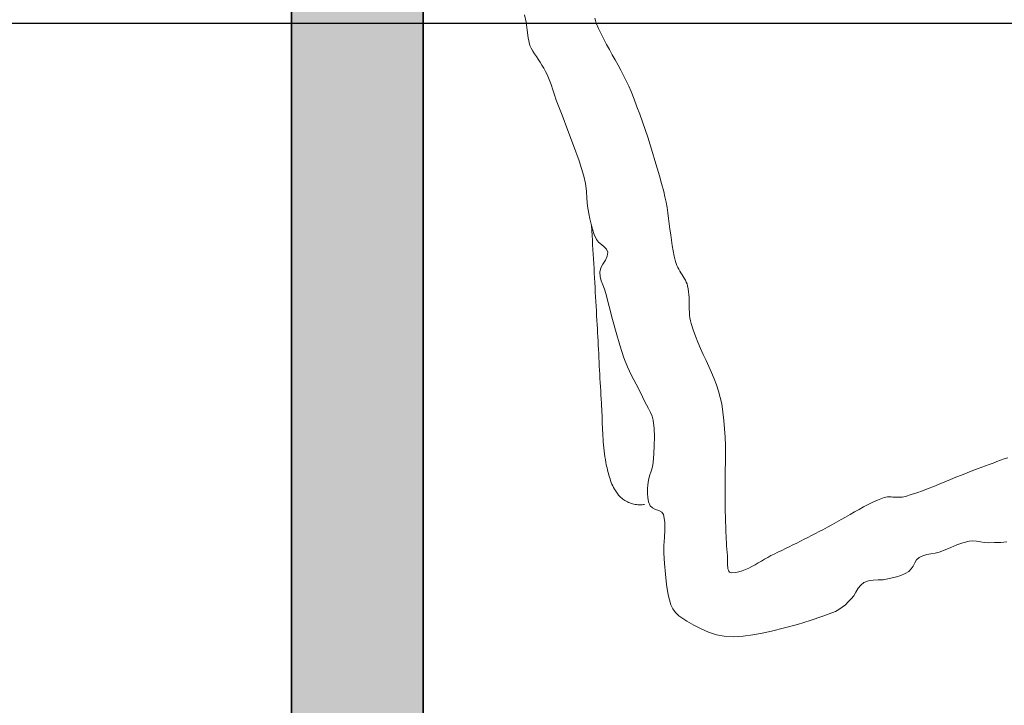
# Model space of a CAD drawing. Units: inches. Extents: x 2656 to 9931, y 1941 to 3068.
# Tile 15 of 46: x 2863 to 2896, y 2466 to 2490. Entities that reach past the tile are written whole.
import ezdxf

# ---------------------------------------------------------------- set-up
doc = ezdxf.new("R2010")
doc.units = ezdxf.units.IN
for name, color, linetype, lineweight in [('A-ANNO-DIMS', 2, 'Continuous', 18), ('A-FURN', 8, 'Continuous', 13), ('A-WALL', 7, 'Continuous', 35), ('A-WALL-PATT', 251, 'Continuous', 13)]:
    doc.layers.add(name, color=color, linetype=linetype, lineweight=lineweight)
doc.styles.get("Standard").update_dxf_attribs({"font": 'arial.ttf'})
doc.dimstyles.new('ISO-25', dxfattribs={"dimtxt": 6, "dimasz": 2.5, "dimexe": 1.25, "dimexo": 0.625, "dimtad": 1, "dimdec": 0, "dimlunit": 3, "dimtxsty": 'Standard', "dimcen": 2.5, "dimadec": 0, "dimazin": 0, "dimtfac": 1, "dimtdec": 0, "dimtmove": 0, "dimatfit": 3, "dimfxl": 1, "dimarcsym": 0})

# ---------------------------------------------------------------- blocks, each defined once
blk = doc.blocks.new('BED-DOUBLE')
for p, q in [((2.814, 22.253), (2.758, 22.509)), ((2.848, 21.988), (2.814, 22.253)), ((5.181, 22.309), (5.16, 22.395)), ((5.21, 22.225), (5.181, 22.309)), ((5.29, 22.04), (5.21, 22.225)), ((2.883, 21.722), (2.848, 21.988)), ((5.376, 21.857), (5.29, 22.04)), ((5.467, 21.676), (5.376, 21.857)), ((2.944, 21.465), (2.883, 21.722)), ((5.562, 21.498), (5.467, 21.676)), ((2.987, 21.364), (2.944, 21.465)), ((3.042, 21.269), (2.987, 21.364)), ((3.105, 21.176), (3.042, 21.269)), ((5.659, 21.32), (5.562, 21.498)), ((5.758, 21.144), (5.659, 21.32)), ((3.17, 21.085), (3.105, 21.176)), ((3.23, 20.991), (3.17, 21.085)), ((3.294, 20.888), (3.23, 20.991)), ((3.358, 20.785), (3.294, 20.888)), ((5.858, 20.967), (5.758, 21.144)), ((5.956, 20.79), (5.858, 20.967)), ((3.422, 20.681), (3.358, 20.785)), ((3.482, 20.575), (3.422, 20.681)), ((3.535, 20.466), (3.482, 20.575)), ((6.053, 20.612), (5.956, 20.79)), ((6.147, 20.433), (6.053, 20.612)), ((3.605, 20.296), (3.535, 20.466)), ((3.669, 20.123), (3.605, 20.296)), ((6.237, 20.253), (6.147, 20.433)), ((6.322, 20.069), (6.237, 20.253)), ((3.729, 19.948), (3.669, 20.123)), ((3.787, 19.772), (3.729, 19.948)), ((6.401, 19.883), (6.322, 20.069)), ((6.502, 19.627), (6.401, 19.883)), ((3.848, 19.598), (3.787, 19.772)), ((4.042, 19.079), (3.848, 19.598)), ((6.6, 19.369), (6.502, 19.627)), ((6.696, 19.11), (6.6, 19.369)), ((4.241, 18.561), (4.042, 19.079)), ((6.789, 18.85), (6.696, 19.11)), ((6.88, 18.59), (6.789, 18.85)), ((4.437, 18.043), (4.241, 18.561)), ((6.968, 18.328), (6.88, 18.59)), ((7.053, 18.065), (6.968, 18.328)), ((4.623, 17.521), (4.437, 18.043)), ((7.136, 17.802), (7.053, 18.065)), ((4.788, 16.993), (4.623, 17.521)), ((7.217, 17.538), (7.136, 17.802)), ((7.295, 17.273), (7.217, 17.538)), ((7.37, 17.008), (7.295, 17.273)), ((4.842, 16.744), (4.788, 16.993)), ((7.443, 16.742), (7.37, 17.008)), ((4.873, 16.49), (4.842, 16.744)), ((4.894, 16.234), (4.873, 16.49)), ((7.514, 16.475), (7.443, 16.742)), ((7.558, 16.293), (7.514, 16.475)), ((4.918, 15.978), (4.894, 16.234)), ((7.596, 16.111), (7.558, 16.293)), ((4.956, 15.726), (4.918, 15.978)), ((7.628, 15.927), (7.596, 16.111)), ((7.656, 15.742), (7.628, 15.927)), ((4.993, 15.544), (4.956, 15.726)), ((5.035, 15.362), (4.993, 15.544)), ((7.682, 15.557), (7.656, 15.742)), ((7.706, 15.371), (7.682, 15.557)), ((5.084, 15.183), (5.035, 15.362)), ((5.061, 15.137), (5.052, 15.298)), ((5.071, 14.976), (5.061, 15.137)), ((5.144, 15.008), (5.084, 15.183)), ((7.729, 15.185), (7.706, 15.371)), ((7.753, 14.999), (7.729, 15.185)), ((5.08, 14.815), (5.071, 14.976)), ((5.089, 14.653), (5.08, 14.815)), ((5.218, 14.839), (5.144, 15.008)), ((5.29, 14.745), (5.218, 14.839)), ((7.778, 14.814), (7.753, 14.999)), ((7.806, 14.629), (7.778, 14.814)), ((5.098, 14.492), (5.089, 14.653)), ((5.107, 14.331), (5.098, 14.492)), ((5.386, 14.665), (5.29, 14.745)), ((5.486, 14.589), (5.386, 14.665)), ((5.567, 14.505), (5.486, 14.589)), ((5.607, 14.402), (5.567, 14.505)), ((7.837, 14.445), (7.806, 14.629)), ((5.116, 14.17), (5.107, 14.331)), ((5.125, 14.008), (5.116, 14.17)), ((5.44, 13.998), (5.524, 14.129)), ((5.524, 14.129), (5.588, 14.261)), ((5.588, 14.261), (5.607, 14.402)), ((7.874, 14.262), (7.837, 14.445)), ((7.916, 14.08), (7.874, 14.262)), ((5.135, 13.847), (5.125, 14.008)), ((5.144, 13.686), (5.135, 13.847)), ((5.331, 13.725), (5.367, 13.865)), ((5.367, 13.865), (5.44, 13.998)), ((7.937, 14.012), (7.916, 14.08)), ((7.963, 13.946), (7.937, 14.012)), ((7.994, 13.881), (7.963, 13.946)), ((8.029, 13.818), (7.994, 13.881)), ((8.066, 13.756), (8.029, 13.818)), ((5.153, 13.525), (5.144, 13.686)), ((5.162, 13.363), (5.153, 13.525)), ((5.341, 13.575), (5.331, 13.725)), ((5.379, 13.427), (5.341, 13.575)), ((8.105, 13.695), (8.066, 13.756)), ((8.144, 13.633), (8.105, 13.695)), ((8.182, 13.572), (8.144, 13.633)), ((8.219, 13.51), (8.182, 13.572)), ((8.254, 13.447), (8.219, 13.51)), ((5.171, 13.202), (5.162, 13.363)), ((5.18, 13.041), (5.171, 13.202)), ((5.432, 13.282), (5.379, 13.427)), ((5.489, 13.137), (5.432, 13.282)), ((5.538, 12.991), (5.489, 13.137)), ((8.285, 13.382), (8.254, 13.447)), ((8.311, 13.316), (8.285, 13.382)), ((8.332, 13.248), (8.311, 13.316)), ((8.352, 13.151), (8.332, 13.248)), ((8.367, 13.053), (8.352, 13.151)), ((5.189, 12.88), (5.18, 13.041)), ((5.198, 12.718), (5.189, 12.88)), ((5.657, 12.549), (5.538, 12.991)), ((8.376, 12.954), (8.367, 13.053)), ((8.381, 12.855), (8.376, 12.954)), ((8.383, 12.755), (8.381, 12.855)), ((5.207, 12.557), (5.198, 12.718)), ((5.216, 12.396), (5.207, 12.557)), ((5.771, 12.106), (5.657, 12.549)), ((8.384, 12.654), (8.383, 12.755)), ((8.385, 12.554), (8.384, 12.654)), ((8.387, 12.454), (8.385, 12.554)), ((8.39, 12.354), (8.387, 12.454)), ((5.225, 12.235), (5.216, 12.396)), ((5.234, 12.073), (5.225, 12.235)), ((5.888, 11.664), (5.771, 12.106)), ((8.397, 12.255), (8.39, 12.354)), ((8.408, 12.156), (8.397, 12.255)), ((8.425, 12.059), (8.408, 12.156)), ((5.242, 11.932), (5.234, 12.073)), ((5.249, 11.79), (5.242, 11.932)), ((5.257, 11.649), (5.249, 11.79)), ((8.449, 11.963), (8.425, 12.059)), ((8.517, 11.748), (8.449, 11.963)), ((5.264, 11.507), (5.257, 11.649)), ((5.272, 11.366), (5.264, 11.507)), ((6.014, 11.224), (5.888, 11.664)), ((8.595, 11.536), (8.517, 11.748)), ((8.68, 11.326), (8.595, 11.536)), ((5.279, 11.224), (5.272, 11.366)), ((5.286, 11.083), (5.279, 11.224)), ((6.158, 10.79), (6.014, 11.224)), ((8.771, 11.118), (8.68, 11.326)), ((8.865, 10.911), (8.771, 11.118)), ((5.294, 10.941), (5.286, 11.083)), ((5.301, 10.8), (5.294, 10.941)), ((5.309, 10.658), (5.301, 10.8)), ((6.281, 10.487), (6.158, 10.79)), ((8.96, 10.704), (8.865, 10.911)), ((5.316, 10.516), (5.309, 10.658)), ((5.323, 10.375), (5.316, 10.516)), ((6.42, 10.191), (6.281, 10.487)), ((9.055, 10.498), (8.96, 10.704)), ((9.147, 10.291), (9.055, 10.498)), ((5.331, 10.233), (5.323, 10.375)), ((5.339, 10.092), (5.331, 10.233)), ((5.347, 9.95), (5.339, 10.092)), ((6.569, 9.899), (6.42, 10.191)), ((9.235, 10.082), (9.147, 10.291)), ((5.355, 9.809), (5.347, 9.95)), ((5.363, 9.667), (5.355, 9.809)), ((6.72, 9.607), (6.569, 9.899)), ((9.315, 9.872), (9.235, 10.082)), ((9.387, 9.659), (9.315, 9.872)), ((5.371, 9.526), (5.363, 9.667)), ((5.38, 9.384), (5.371, 9.526)), ((6.864, 9.313), (6.72, 9.607)), ((9.447, 9.442), (9.387, 9.659)), ((9.495, 9.223), (9.447, 9.442)), ((5.389, 9.243), (5.38, 9.384)), ((5.395, 9.142), (5.389, 9.243)), ((5.4, 9.04), (5.395, 9.142)), ((6.93, 9.186), (6.864, 9.313)), ((7, 9.061), (6.93, 9.186)), ((9.539, 8.941), (9.495, 9.223)), ((5.404, 8.939), (5.4, 9.04)), ((5.408, 8.837), (5.404, 8.939)), ((5.412, 8.735), (5.408, 8.837)), ((7.067, 8.934), (7, 9.061)), ((7.122, 8.804), (7.067, 8.934)), ((7.155, 8.667), (7.122, 8.804)), ((9.573, 8.659), (9.539, 8.941)), ((5.416, 8.634), (5.412, 8.735)), ((5.419, 8.532), (5.416, 8.634)), ((5.423, 8.43), (5.419, 8.532)), ((5.427, 8.329), (5.423, 8.43)), ((7.184, 8.38), (7.155, 8.667)), ((9.596, 8.375), (9.573, 8.659)), ((5.432, 8.227), (5.427, 8.329)), ((5.437, 8.125), (5.432, 8.227)), ((5.443, 8.024), (5.437, 8.125)), ((7.195, 8.092), (7.184, 8.38)), ((7.192, 7.802), (7.195, 8.092)), ((9.611, 8.09), (9.596, 8.375)), ((9.62, 7.805), (9.611, 8.09)), ((5.45, 7.923), (5.443, 8.024)), ((5.458, 7.822), (5.45, 7.923)), ((5.468, 7.721), (5.458, 7.822)), ((7.178, 7.513), (7.192, 7.802)), ((9.622, 7.519), (9.62, 7.805)), ((5.479, 7.62), (5.468, 7.721)), ((5.492, 7.52), (5.479, 7.62)), ((5.506, 7.419), (5.492, 7.52)), ((5.522, 7.319), (5.506, 7.419)), ((7.156, 7.225), (7.178, 7.513)), ((9.621, 7.233), (9.622, 7.519)), ((5.541, 7.22), (5.522, 7.319)), ((5.553, 7.158), (5.541, 7.22)), ((5.566, 7.096), (5.553, 7.158)), ((5.58, 7.034), (5.566, 7.096)), ((7.085, 6.92), (7.129, 7.071)), ((7.129, 7.071), (7.156, 7.225)), ((9.618, 6.946), (9.621, 7.233)), ((18.509, 7.107), (18.383, 7.06)), ((18.634, 7.155), (18.509, 7.107)), ((18.76, 7.204), (18.634, 7.155)), ((18.885, 7.251), (18.76, 7.204)), ((19.011, 7.298), (18.885, 7.251)), ((19.137, 7.343), (19.011, 7.298)), ((19.264, 7.386), (19.137, 7.343)), ((5.594, 6.972), (5.58, 7.034)), ((5.609, 6.909), (5.594, 6.972)), ((5.626, 6.847), (5.609, 6.909)), ((5.643, 6.785), (5.626, 6.847)), ((5.661, 6.724), (5.643, 6.785)), ((6.992, 6.618), (7.035, 6.769)), ((7.035, 6.769), (7.085, 6.92)), ((9.614, 6.66), (9.618, 6.946)), ((17.684, 6.794), (17.494, 6.717)), ((17.874, 6.869), (17.684, 6.794)), ((18.066, 6.943), (17.874, 6.869)), ((18.258, 7.014), (18.066, 6.943)), ((18.383, 7.06), (18.258, 7.014)), ((5.681, 6.663), (5.661, 6.724)), ((5.702, 6.603), (5.681, 6.663)), ((5.725, 6.543), (5.702, 6.603)), ((5.749, 6.484), (5.725, 6.543)), ((5.776, 6.427), (5.749, 6.484)), ((5.804, 6.37), (5.776, 6.427)), ((6.96, 6.317), (6.968, 6.464)), ((6.968, 6.464), (6.992, 6.618)), ((9.611, 6.373), (9.614, 6.66)), ((16.735, 6.407), (16.545, 6.332)), ((16.925, 6.483), (16.735, 6.407)), ((17.115, 6.561), (16.925, 6.483)), ((17.304, 6.639), (17.115, 6.561)), ((17.494, 6.717), (17.304, 6.639)), ((5.833, 6.315), (5.804, 6.37)), ((5.865, 6.261), (5.833, 6.315)), ((5.899, 6.209), (5.865, 6.261)), ((5.936, 6.159), (5.899, 6.209)), ((5.975, 6.11), (5.936, 6.159)), ((6.016, 6.063), (5.975, 6.11)), ((6.047, 6.031), (6.016, 6.063)), ((6.959, 6.168), (6.96, 6.317)), ((6.97, 6.021), (6.959, 6.168)), ((9.609, 6.087), (9.611, 6.373)), ((9.612, 5.801), (9.609, 6.087)), ((15.773, 6.06), (15.714, 6.046)), ((15.968, 6.123), (15.773, 6.06)), ((16.161, 6.189), (15.968, 6.123)), ((16.354, 6.259), (16.161, 6.189)), ((16.545, 6.332), (16.354, 6.259)), ((6.081, 6.001), (6.047, 6.031)), ((6.116, 5.972), (6.081, 6.001)), ((6.154, 5.945), (6.116, 5.972)), ((6.193, 5.92), (6.154, 5.945)), ((6.233, 5.897), (6.193, 5.92)), ((6.275, 5.876), (6.233, 5.897)), ((6.318, 5.856), (6.275, 5.876)), ((6.362, 5.839), (6.318, 5.856)), ((6.407, 5.823), (6.362, 5.839)), ((6.452, 5.81), (6.407, 5.823)), ((6.498, 5.798), (6.452, 5.81)), ((6.544, 5.789), (6.498, 5.798)), ((6.591, 5.783), (6.544, 5.789)), ((6.637, 5.778), (6.591, 5.783)), ((6.684, 5.776), (6.637, 5.778)), ((6.73, 5.776), (6.684, 5.776)), ((6.775, 5.779), (6.73, 5.776)), ((6.82, 5.784), (6.775, 5.779)), ((6.864, 5.792), (6.82, 5.784)), ((7, 5.878), (6.97, 6.021)), ((7.054, 5.745), (7, 5.878)), ((7.129, 5.669), (7.054, 5.745)), ((9.619, 5.515), (9.612, 5.801)), ((14.501, 5.787), (14.343, 5.705)), ((14.66, 5.864), (14.501, 5.787)), ((14.821, 5.938), (14.66, 5.864)), ((14.984, 6.007), (14.821, 5.938)), ((15.041, 6.026), (14.984, 6.007)), ((15.1, 6.038), (15.041, 6.026)), ((15.16, 6.045), (15.1, 6.038)), ((15.221, 6.047), (15.16, 6.045)), ((15.282, 6.046), (15.221, 6.047)), ((15.344, 6.043), (15.282, 6.046)), ((15.407, 6.039), (15.344, 6.043)), ((15.469, 6.035), (15.407, 6.039)), ((15.531, 6.033), (15.469, 6.035)), ((15.593, 6.033), (15.531, 6.033)), ((15.654, 6.037), (15.593, 6.033)), ((15.714, 6.046), (15.654, 6.037)), ((7.236, 5.621), (7.129, 5.669)), ((7.351, 5.581), (7.236, 5.621)), ((7.45, 5.529), (7.351, 5.581)), ((7.508, 5.447), (7.45, 5.529)), ((7.553, 5.189), (7.508, 5.447)), ((9.623, 5.402), (9.619, 5.515)), ((9.627, 5.288), (9.623, 5.402)), ((13.878, 5.447), (13.724, 5.359)), ((14.032, 5.535), (13.878, 5.447)), ((14.187, 5.621), (14.032, 5.535)), ((14.343, 5.705), (14.187, 5.621)), ((7.556, 4.925), (7.553, 5.189)), ((9.63, 5.174), (9.627, 5.288)), ((9.633, 5.061), (9.63, 5.174)), ((9.636, 4.947), (9.633, 5.061)), ((13.261, 5.095), (13.106, 5.009)), ((13.416, 5.182), (13.261, 5.095)), ((13.57, 5.27), (13.416, 5.182)), ((13.724, 5.359), (13.57, 5.27)), ((7.538, 4.658), (7.556, 4.925)), ((9.64, 4.833), (9.636, 4.947)), ((9.644, 4.72), (9.64, 4.833)), ((9.648, 4.606), (9.644, 4.72)), ((12.567, 4.73), (12.44, 4.665)), ((12.695, 4.795), (12.567, 4.73)), ((12.822, 4.861), (12.695, 4.795)), ((12.949, 4.926), (12.822, 4.861)), ((13.106, 5.009), (12.949, 4.926)), ((7.52, 4.39), (7.538, 4.658)), ((7.523, 4.124), (7.52, 4.39)), ((9.654, 4.493), (9.648, 4.606)), ((9.661, 4.379), (9.654, 4.493)), ((9.669, 4.266), (9.661, 4.379)), ((11.929, 4.408), (11.801, 4.344)), ((12.057, 4.472), (11.929, 4.408)), ((12.185, 4.536), (12.057, 4.472)), ((12.313, 4.6), (12.185, 4.536)), ((12.44, 4.665), (12.313, 4.6)), ((17.526, 4.406), (17.324, 4.323)), ((17.73, 4.479), (17.526, 4.406)), ((17.94, 4.533), (17.73, 4.479)), ((18.07, 4.542), (17.94, 4.533)), ((18.2, 4.53), (18.07, 4.542)), ((18.331, 4.508), (18.2, 4.53)), ((18.463, 4.487), (18.331, 4.508)), ((18.594, 4.48), (18.463, 4.487)), ((18.808, 4.485), (18.594, 4.48)), ((19.022, 4.492), (18.808, 4.485)), ((19.236, 4.507), (19.022, 4.492)), ((7.547, 3.768), (7.523, 4.124)), ((9.678, 4.153), (9.669, 4.266)), ((9.69, 4.04), (9.678, 4.153)), ((9.693, 3.991), (9.69, 4.04)), ((11.176, 4.041), (11.068, 3.982)), ((11.286, 4.096), (11.176, 4.041)), ((11.415, 4.157), (11.286, 4.096)), ((11.544, 4.219), (11.415, 4.157)), ((11.672, 4.281), (11.544, 4.219)), ((11.801, 4.344), (11.672, 4.281)), ((16.362, 4.037), (16.236, 3.976)), ((16.497, 4.076), (16.362, 4.037)), ((16.638, 4.103), (16.497, 4.076)), ((16.78, 4.129), (16.638, 4.103)), ((16.918, 4.164), (16.78, 4.129)), ((17.123, 4.239), (16.918, 4.164)), ((17.324, 4.323), (17.123, 4.239)), ((7.571, 3.41), (7.547, 3.768)), ((9.694, 3.937), (9.693, 3.991)), ((9.694, 3.879), (9.694, 3.937)), ((9.694, 3.819), (9.694, 3.879)), ((9.694, 3.759), (9.694, 3.819)), ((9.696, 3.701), (9.694, 3.759)), ((9.701, 3.645), (9.696, 3.701)), ((10.636, 3.73), (10.528, 3.671)), ((10.745, 3.793), (10.636, 3.73)), ((10.852, 3.856), (10.745, 3.793)), ((10.96, 3.92), (10.852, 3.856)), ((11.068, 3.982), (10.96, 3.92)), ((16.088, 3.796), (16.032, 3.687)), ((16.152, 3.897), (16.088, 3.796)), ((16.236, 3.976), (16.152, 3.897)), ((7.605, 3.054), (7.571, 3.41)), ((9.71, 3.593), (9.701, 3.645)), ((9.723, 3.548), (9.71, 3.593)), ((9.741, 3.51), (9.723, 3.548)), ((9.767, 3.482), (9.741, 3.51)), ((9.8, 3.464), (9.767, 3.482)), ((9.841, 3.459), (9.8, 3.464)), ((9.961, 3.47), (9.841, 3.459)), ((10.078, 3.492), (9.961, 3.47)), ((10.193, 3.525), (10.078, 3.492)), ((10.306, 3.567), (10.193, 3.525)), ((10.418, 3.616), (10.306, 3.567)), ((10.528, 3.671), (10.418, 3.616)), ((15.615, 3.368), (15.469, 3.321)), ((15.756, 3.427), (15.615, 3.368)), ((15.887, 3.503), (15.756, 3.427)), ((15.969, 3.585), (15.887, 3.503)), ((16.032, 3.687), (15.969, 3.585)), ((7.663, 2.703), (7.605, 3.054)), ((14.241, 3.037), (14.156, 2.925)), ((14.35, 3.122), (14.241, 3.037)), ((14.503, 3.18), (14.35, 3.122)), ((14.667, 3.204), (14.503, 3.18)), ((14.836, 3.212), (14.667, 3.204)), ((15.006, 3.22), (14.836, 3.212)), ((15.171, 3.245), (15.006, 3.22)), ((15.32, 3.282), (15.171, 3.245)), ((15.469, 3.321), (15.32, 3.282)), ((7.755, 2.361), (7.663, 2.703)), ((14.081, 2.799), (14.006, 2.674)), ((14.156, 2.925), (14.081, 2.799)), ((7.822, 2.221), (7.755, 2.361)), ((13.719, 2.367), (13.613, 2.277)), ((13.819, 2.464), (13.719, 2.367)), ((13.917, 2.562), (13.819, 2.464)), ((14.006, 2.674), (13.917, 2.562)), ((7.918, 2.097), (7.822, 2.221)), ((8.036, 1.988), (7.918, 2.097)), ((13.378, 2.137), (12.951, 1.974)), ((13.5, 2.198), (13.378, 2.137)), ((13.613, 2.277), (13.5, 2.198)), ((8.166, 1.891), (8.036, 1.988)), ((8.301, 1.807), (8.166, 1.891)), ((8.543, 1.669), (8.301, 1.807)), ((12.081, 1.691), (11.64, 1.572)), ((12.518, 1.825), (12.081, 1.691)), ((12.951, 1.974), (12.518, 1.825)), ((8.793, 1.539), (8.543, 1.669)), ((9.05, 1.427), (8.793, 1.539)), ((9.313, 1.341), (9.05, 1.427)), ((10.877, 1.396), (10.555, 1.334)), ((11.195, 1.465), (10.877, 1.396)), ((11.64, 1.572), (11.195, 1.465)), ((9.585, 1.289), (9.313, 1.341)), ((9.908, 1.271), (9.585, 1.289)), ((10.231, 1.29), (9.908, 1.271)), ((10.555, 1.334), (10.231, 1.29))]:
    blk.add_line(p, q)
blk = doc.blocks.new('*D31')
at = {"layer": 'A-ANNO-DIMS', "color": 0, "lineweight": -2, "transparency": 16777216}
for p, q in [((2753.358, 2502.145), (2753.358, 2488.227)), ((2841.982, 2502.145), (2841.982, 2488.227)), ((2755.858, 2489.477), (2839.482, 2489.477)), ((2841.982, 2489.477), (2952.348, 2489.477))]:
    blk.add_line(p, q, dxfattribs=at)
at = {"layer": 'A-ANNO-DIMS', "color": 0, "transparency": 16777216}
for points in [[(2755.858, 2489.893), (2755.858, 2489.06), (2753.358, 2489.477)], [(2839.482, 2489.893), (2839.482, 2489.06), (2841.982, 2489.477)]]:
    blk.add_solid(points, dxfattribs=at)
at = {"layer": 'Defpoints', "color": 0, "transparency": 16777216}
for p in [(2753.358, 2502.77), (2841.982, 2502.77), (2841.982, 2489.477)]:
    blk.add_point(p, dxfattribs=at)
at = {"layer": 'A-ANNO-DIMS', "color": 0, "transparency": 16777216, "insert": (2898.415, 2493.206), "char_height": 6, "attachment_point": 5}
blk.add_mtext('DOUBLE BED 7\'-4 1/2" TYP.', dxfattribs=at)
blk = doc.blocks.new('*D102')
at = {"layer": 'A-ANNO-DIMS', "color": 0, "lineweight": -2, "transparency": 16777216}
for p, q in [((2998.157, 2604.975), (2998.157, 2009.273)), ((2872.157, 2564.712), (2872.157, 2009.273)), ((2874.657, 2010.523), (2995.657, 2010.523))]:
    blk.add_line(p, q, dxfattribs=at)
at = {"layer": 'A-ANNO-DIMS', "color": 0, "transparency": 16777216}
for points in [[(2874.657, 2010.939), (2874.657, 2010.106), (2872.157, 2010.523)], [(2995.657, 2010.939), (2995.657, 2010.106), (2998.157, 2010.523)]]:
    blk.add_solid(points, dxfattribs=at)
at = {"layer": 'Defpoints', "color": 0, "transparency": 16777216}
for p in [(2998.157, 2605.6), (2872.157, 2565.337), (2998.157, 2010.523)]:
    blk.add_point(p, dxfattribs=at)
at = {"layer": 'A-ANNO-DIMS', "color": 0, "transparency": 16777216, "insert": (2935.157, 2014.211), "char_height": 6, "attachment_point": 5}
blk.add_mtext('10\'-6"', dxfattribs=at)

msp = doc.modelspace()

# ---------------------------------------------------------------- hatches: boundary and pattern name
at = {"layer": 'A-WALL-PATT'}
h = msp.add_hatch(color=256, dxfattribs=at)
h.dxf.hatch_style = 1
h.paths.add_polyline_path([(2858.657, 2623.6), (2752.157, 2623.6), (2752.157, 2614.6), (2858.657, 2614.6)])
h.paths.add_polyline_path([(2893.087, 2623.6), (2876.657, 2623.6), (2876.657, 2614.6), (2893.087, 2614.6), (2893.087, 2619.1)])
h.paths.add_polyline_path([(2946.514, 2623.6), (2917.087, 2623.6), (2917.087, 2614.6), (2946.514, 2614.6), (2946.514, 2619.1)])
h.paths.add_polyline_path([(2989.157, 2623.6), (2970.514, 2623.6), (2970.514, 2614.6), (2989.157, 2614.6)])
h.paths.add_polyline_path([(2998.157, 2605.6), (2989.157, 2605.6), (2989.157, 2523.881), (2998.157, 2523.881)])
h.paths.add_polyline_path([(2935.157, 2614.6), (2930.657, 2614.6), (2930.657, 2554.6), (2876.657, 2554.6), (2876.657, 2565.337), (2872.157, 2565.337), (2872.157, 2444.1), (2876.657, 2444.1), (2876.657, 2550.1), (2946.472, 2550.1), (2946.472, 2554.6), (2935.157, 2554.6)])
h.paths.add_polyline_path([(2989.157, 2554.6), (2982.11, 2554.6), (2976.574, 2554.6), (2976.574, 2550.1), (2982.11, 2550.1), (2989.157, 2550.1)])
h.paths.add_polyline_path([(2876.657, 2614.6), (2872.157, 2614.6), (2872.157, 2595.003), (2876.657, 2595.003)], flags=0)
h.paths.add_polyline_path([(2752.157, 2605.6), (2743.157, 2605.6), (2743.157, 2544.033), (2752.157, 2544.033)])
h.paths.add_polyline_path([(2752.157, 2426.1), (2743.157, 2426.1), (2743.157, 2300.1), (2752.157, 2300.1)])
h.paths.add_polyline_path([(2821.134, 2430.6), (2752.157, 2430.6), (2752.157, 2426.1), (2821.134, 2426.1)])
h.paths.add_polyline_path([(2867.657, 2430.6), (2862.876, 2430.6), (2862.876, 2426.1), (2867.657, 2426.1)])
h.paths.add_polyline_path([(2752.157, 2484.033), (2747.657, 2484.033), (2743.157, 2484.033), (2743.157, 2444.1), (2752.157, 2444.1)])
h.paths.add_polyline_path([(2998.157, 2426.1), (2989.157, 2426.1), (2989.157, 2390.1), (2872.157, 2390.1), (2872.157, 2385.6), (2876.657, 2385.6), (2989.157, 2385.6), (2989.157, 2365.037), (2998.157, 2365.037)])
h.paths.add_polyline_path([(2998.157, 2463.881), (2993.657, 2463.881), (2989.157, 2463.881), (2989.157, 2444.1), (2998.157, 2444.1)])
h.paths.add_polyline_path([(2998.157, 2319.88), (2989.157, 2319.88), (2989.157, 2300.1), (2998.157, 2300.1)])
h.paths.add_polyline_path([(2998.157, 2282.1), (2989.157, 2282.1), (2989.157, 2253.6), (2982.058, 2253.6), (2982.058, 2249.1), (2989.157, 2249.1), (2998.157, 2249.1)])
h.paths.add_polyline_path([(2931.542, 2253.6), (2923.796, 2253.6), (2923.796, 2249.1), (2931.542, 2249.1)])
h.paths.add_polyline_path([(2876.657, 2282.1), (2872.157, 2282.1), (2872.157, 2184.6), (2872.157, 2175.6), (2876.657, 2175.6), (2876.657, 2249.1), (2888.323, 2249.1), (2888.323, 2251.35), (2888.323, 2253.6), (2876.657, 2253.6)])
h.paths.add_polyline_path([(2858.657, 2175.6), (2841.419, 2175.6), (2841.419, 2166.6), (2858.657, 2166.6)])
h.paths.add_polyline_path([(2785.058, 2171.1), (2785.058, 2175.6), (2752.157, 2175.6), (2752.157, 2166.6), (2785.058, 2166.6)])
h.paths.add_polyline_path([(2752.157, 2282.1), (2743.157, 2282.1), (2743.157, 2184.6), (2752.157, 2184.6)])
h.paths.add_polyline_path([(2809.769, 2300.1), (2752.157, 2300.1), (2752.157, 2295.6), (2809.769, 2295.6)])
h.paths.add_polyline_path([(2867.657, 2300.1), (2851.877, 2300.1), (2851.877, 2295.6), (2867.657, 2295.6)])

# ---------------------------------------------------------------- linework, layer by layer
at = {"layer": 'A-WALL'}
for p, q in [((2872.157, 2565.337), (2872.157, 2444.1)), ((2876.657, 2550.1), (2876.657, 2426.1))]:
    msp.add_line(p, q, dxfattribs=at)

# ---------------------------------------------------------------- block references
at = {"layer": 'A-FURN'}
msp.add_blockref('BED-DOUBLE', (2877.353, 2467.251), dxfattribs=at)

# ---------------------------------------------------------------- dimensions: what is measured, and where the dimension line sits
at = {"layer": 'A-ANNO-DIMS'}
dim = msp.add_linear_dim(base=(2998.157, 2010.523), p1=(2872.157, 2565.337), p2=(2998.157, 2605.6), dimstyle='ISO-25', override={"dimdec": 1, "dimlfac": 1, "dimrnd": 0, "dimzin": 1, "dimdsep": 46, "dimlunit": 4, "dimfrac": 2}, dxfattribs=at)
dim.commit()
dim.dimension.update_dxf_attribs({"geometry": '*D102', "text_midpoint": (2935.157, 2014.211)})
dim = msp.add_linear_dim(base=(2841.982, 2489.477), p1=(2753.358, 2502.77), p2=(2841.982, 2502.77), text='DOUBLE BED <> TYP.', dimstyle='ISO-25', override={"dimdec": 1, "dimlfac": 1, "dimrnd": 0, "dimzin": 1, "dimdsep": 46, "dimlunit": 4, "dimfrac": 2}, dxfattribs=at)
dim.commit()
dim.dimension.update_dxf_attribs({"geometry": '*D31', "text_midpoint": (2898.415, 2493.206)})

doc.saveas('drawing.dxf')
